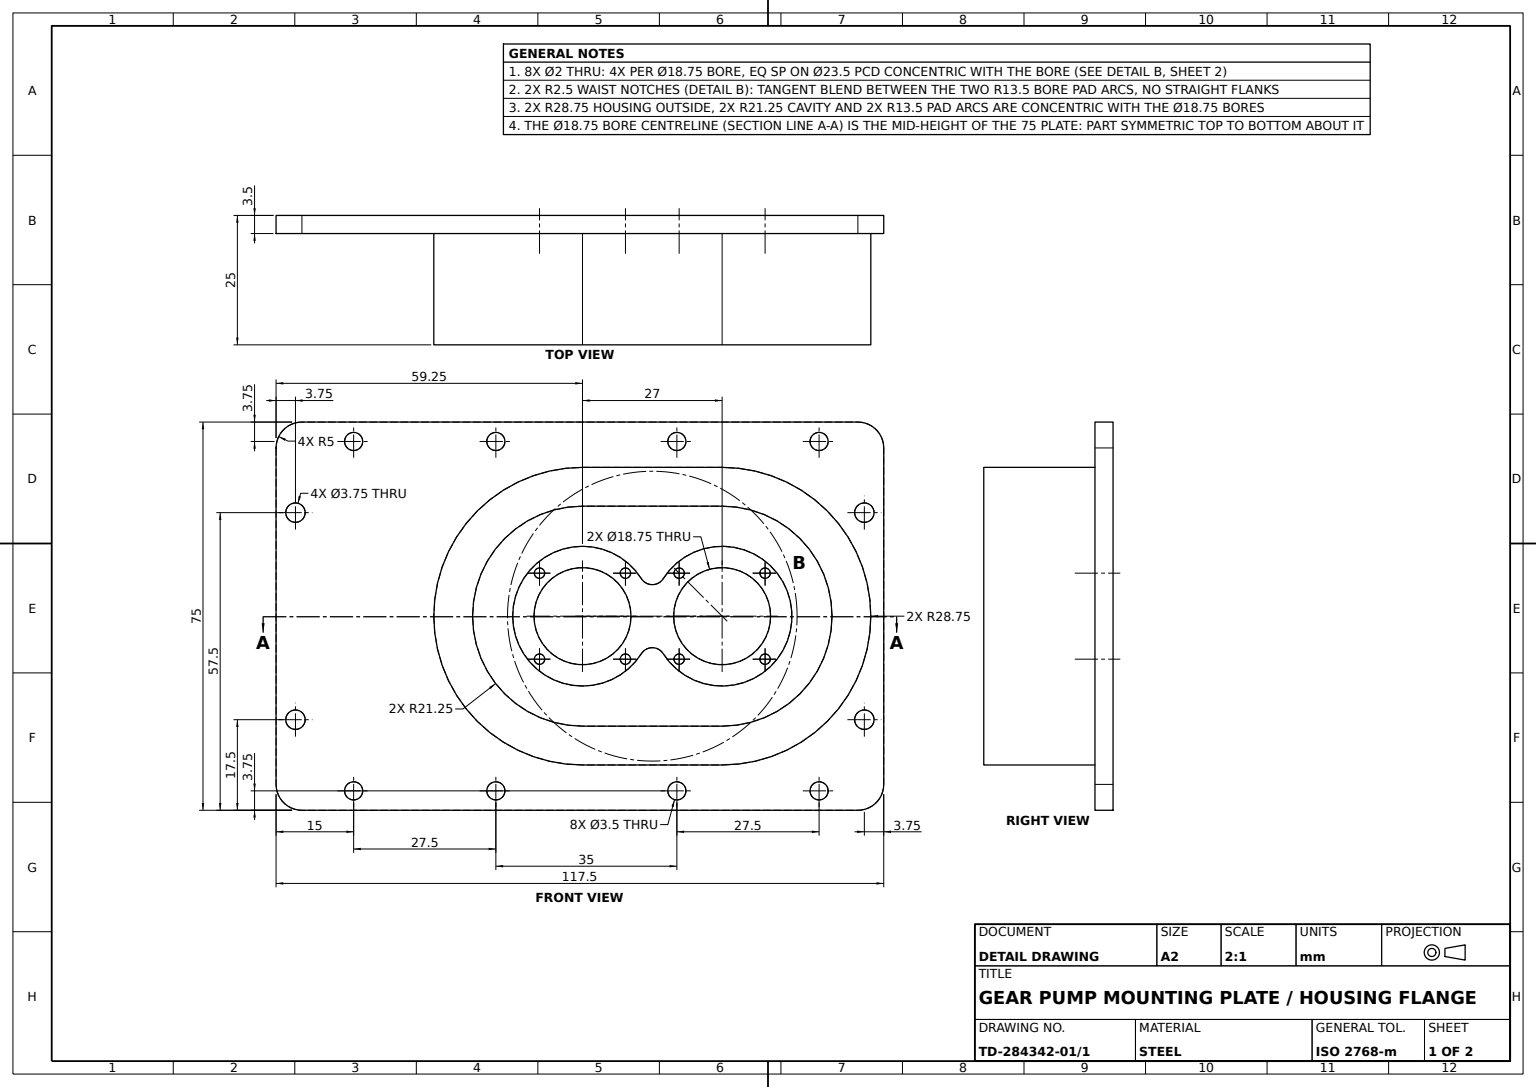
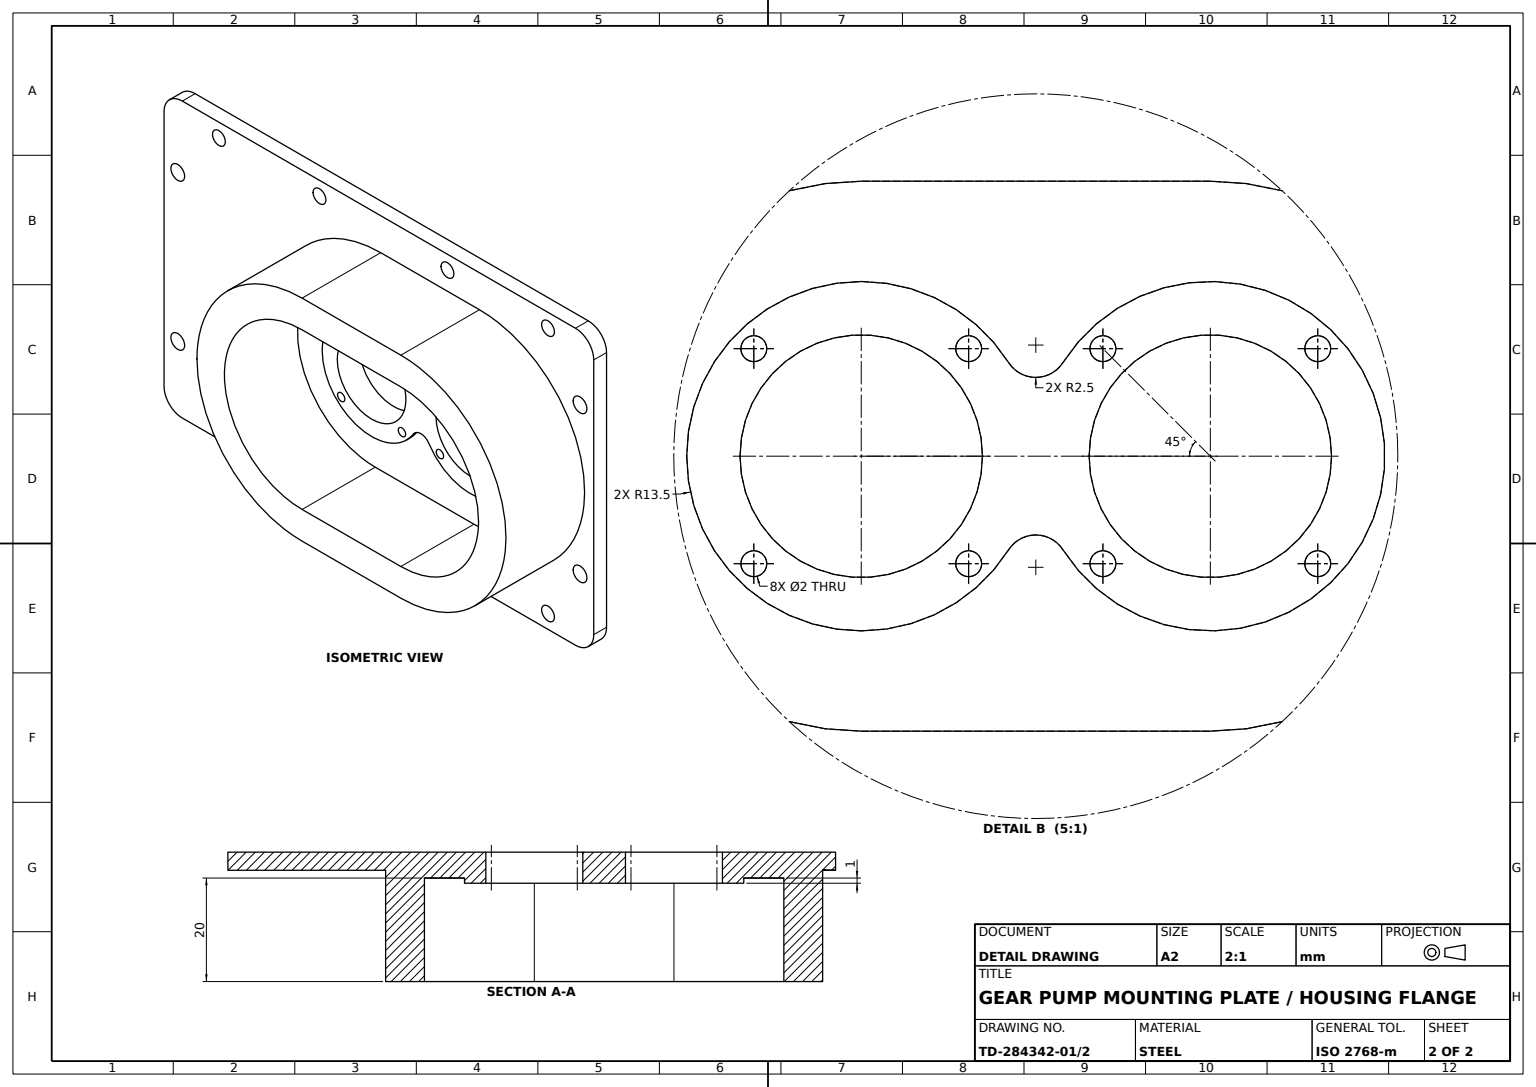
SolidWorks part; units mm, degrees
material "Plain Carbon Steel"
ref_plane "Front Plane" through (0, 0, 0) normal (0, 0, 1) x (1, 0, 0)
ref_plane "Top Plane" through (0, 0, 0) normal (0, 1, 0) x (1, 0, 0)
ref_plane "Right Plane" through (0, 0, 0) normal (1, 0, 0) x (0, 0, -1)
sketch "Flange Plate Sketch" plane through (0, 0, 0) normal (0, 0, 1) x (1, 0, 0)
  line L0 (0, 0) -> (117.5, 0)
  line L1 (117.5, 0) -> (117.5, 75)
  line L2 (117.5, 75) -> (0, 75)
  line L3 (0, 75) -> (0, 0)
  dimension "D1" = 117.5
  dimension "D2" = 75
extrude "Flange Plate" add sketch "Flange Plate Sketch" along normal blind 3.5
sketch "Housing Wall Sketch" plane through (0, 0, 3.5) normal (0, 0, 1) x (1, 0, 0)
  line L0 (0, 37.5) -> (59.25, 37.5) construction
  line L1 (0, 75) -> (0, 0) construction
  line L2 (59.25, 37.5) -> (86.25, 37.5) construction
  line L3 (59.25, 37.5) -> (86.25, 37.5) construction
  line L4 (59.25, 66.25) -> (86.25, 66.25)
  line L5 (59.25, 8.75) -> (86.25, 8.75)
  arc A0 (59.25, 66.25) -> (59.25, 8.75) centre (59.25, 37.5) ccw
  arc A1 (86.25, 8.75) -> (86.25, 66.25) centre (86.25, 37.5) ccw
  point P5 (72.75, 37.5)
  dimension "D1" = 28.75
  dimension "D2" = 59.25
  dimension "D3" = 72.75
extrude "Housing Wall" add sketch "Housing Wall Sketch" along normal blind 21.5
sketch "Housing Cavity Sketch" plane through (0, 0, 25) normal (0, 0, 1) x (1, 0, 0)
  line L0 (86.25, 37.5) -> (59.25, 37.5) construction
  line L1 (86.25, 16.25) -> (59.25, 16.25)
  line L2 (86.25, 58.75) -> (59.25, 58.75)
  arc A0 (86.25, 16.25) -> (86.25, 58.75) centre (86.25, 37.5) ccw
  arc A1 (59.25, 58.75) -> (59.25, 16.25) centre (59.25, 37.5) ccw
  point P2 (72.75, 37.5)
  dimension "D1" = 21.25
extrude "Housing Cavity" cut sketch "Housing Cavity Sketch" against normal blind 20
sketch "Dual Bore Sketch" plane through (0, 0, 5) normal (0, 0, 1) x (1, 0, 0)
  line L0 (59.25, 37.5) -> (86.25, 37.5) construction
  circle A0 centre (59.25, 37.5) radius 9.375
  circle A1 centre (86.25, 37.5) radius 9.375
  dimension "D1" = 18.75
  dimension "D2" = 18.75
extrude "Dual Bores" cut sketch "Dual Bore Sketch" against normal through all
sketch "Bore Pad Sketch" plane through (0, 0, 5) normal (0, 0, 1) x (1, 0, 0)
  line L0 (59.25, 37.5) -> (86.25, 37.5) construction
  arc A0 (70.6406, 44.7459) -> (70.6406, 30.2541) centre (59.25, 37.5) ccw
  arc A1 (74.8594, 30.2541) -> (74.8594, 44.7459) centre (86.25, 37.5) ccw
  circle A2 centre (59.25, 37.5) radius 9.375
  circle A3 centre (86.25, 37.5) radius 9.375
  arc A4 (70.6406, 44.7459) -> (74.8594, 44.7459) centre (72.75, 46.0878) ccw
  arc A5 (74.8594, 30.2541) -> (70.6406, 30.2541) centre (72.75, 28.9122) ccw
  dimension "D1" = 27
  dimension "D2" = 27
  dimension "D3" = 18.75
  dimension "D4" = 18.75
  dimension "D5" = 5
  dimension "D6" = 5
extrude "Bore Pads" add sketch "Bore Pad Sketch" along normal blind 1
sketch "Bore Slot Sketch" plane through (0, 0, 6) normal (0, 0, 1) x (1, 0, 0)
  line L0 (45.75, 37.5) -> (99.75, 37.5) construction
  line L1 (59.25, 37.5) -> (67.5585, 29.1915) construction
  circle A0 centre (59.25, 37.5) radius 11.75 construction
  circle A1 centre (86.25, 37.5) radius 11.75 construction
  arc A2 (70.6406, 44.7459) -> (70.6406, 30.2541) centre (59.25, 37.5) ccw construction
  arc A3 (74.8594, 30.2541) -> (74.8594, 44.7459) centre (86.25, 37.5) ccw construction
  circle A4 centre (67.5585, 29.1915) radius 1
  dimension "D1" = 23.5
  dimension "D2" = 23.5
  dimension "D4" = 2
  dimension "D3" = 45
extrude "Bore Slot Cut" cut sketch "Bore Slot Sketch" against normal through all
pattern_circular "Bore Slot Pattern 4x" count 4 over 360 about axis through (59.25, 37.5, 0) along (0, 0, 1) of "Bore Slot Cut"
sketch "Bore Notch Sketch" plane through (0, 0, 6) normal (0, 0, 1) x (1, 0, 0)
  line L0 (86.25, 37.5) -> (98, 37.5) construction
  line L1 (86.25, 37.5) -> (94.5585, 29.1915) construction
  circle A0 centre (86.25, 37.5) radius 11.75 construction
  circle A1 centre (94.5585, 29.1915) radius 1
  dimension "D1" = 23.5
  dimension "D2" = 45
  dimension "D3" = 2
extrude "Bore Notch Cut" cut sketch "Bore Notch Sketch" against normal through all
pattern_circular "Bore Notch Pattern 4x" count 4 over 360 about axis through (86.25, 37.5, 0) along (0, 0, 1) of "Bore Notch Cut"
fillet "Flange Corner Fillets R5" radius 5 4 edges at (0, 0, 1.75) (117.5, 0, 1.75) (117.5, 75, 1.75) (0, 75, 1.75)
sketch "Flange Edge Hole Sketch" plane through (0, 0, 3.5) normal (0, 0, 1) x (1, 0, 0)
  line L0 (112.5, 75) -> (5, 75) construction
  circle A0 centre (15, 71.25) radius 1.75
  dimension "D1" = 3.5
  dimension "D2" = 3.75
  dimension "D3" = 10
extrude "Flange Edge Hole" cut sketch "Flange Edge Hole Sketch" against normal through all
pattern_linear "Flange Edge Hole Pattern" count 2 spacing 27.5 along (1, 0, 0) of "Flange Edge Hole"
sketch "Flange Side Hole Sketch" plane through (0, 0, 3.5) normal (0, 0, 1) x (1, 0, 0)
  line L0 (112.5, 75) -> (5, 75) construction
  line L1 (42.5, 73) -> (42.5, 69.5) construction
  line L2 (44.25, 71.25) -> (40.75, 71.25) construction
  circle A0 centre (77.5, 71.25) radius 1.75
  circle A1 centre (105, 71.25) radius 1.75
  circle A2 centre (42.5, 71.25) radius 1.75 construction
  point P13 (42.5, 71.25)
  dimension "D1" = 3.5
  dimension "D2" = 3.5
  dimension "D3" = 3.75
  dimension "D4" = 3.75
  dimension "D5" = 35
  dimension "D6" = 27.5
extrude "Flange Side Holes" cut sketch "Flange Side Hole Sketch" against normal through all
sketch "Flange Corner Hole Sketch" plane through (0, 0, 3.5) normal (0, 0, 1) x (1, 0, 0)
  line L0 (117.5, 5) -> (117.5, 70) construction
  line L1 (117.5, 37.5) -> (115, 37.5) construction
  circle A0 centre (113.75, 57.5) radius 1.875
  circle A1 centre (113.75, 17.5) radius 1.875
  arc A2 (86.25, 8.75) -> (86.25, 66.25) centre (86.25, 37.5) ccw construction
  dimension "D1" = 3.75
  dimension "D2" = 3.75
  dimension "D3" = 3.75
  dimension "D4" = 3.75
  dimension "D5" = 20
  dimension "D6" = 20
extrude "Flange Corner Holes" cut sketch "Flange Corner Hole Sketch" against normal through all
ref_plane "Flange Hole Mirror Plane" through (0, 37.5, 0) normal (0, 1, 0) x (1, 0, 0)
mirror "Flange Hole Mirror" about plane through (0, 37.5, 0) normal (0, 1, 0) of "Flange Side Holes", "Flange Edge Hole Pattern", "Flange Edge Hole"
ref_plane "Corner Hole Mirror Plane" through (58.75, 0, 0) normal (1, 0, 0) x (0, 0, -1)
mirror "Corner Hole Mirror" about plane through (58.75, 0, 0) normal (1, 0, 0) of "Flange Corner Holes"
